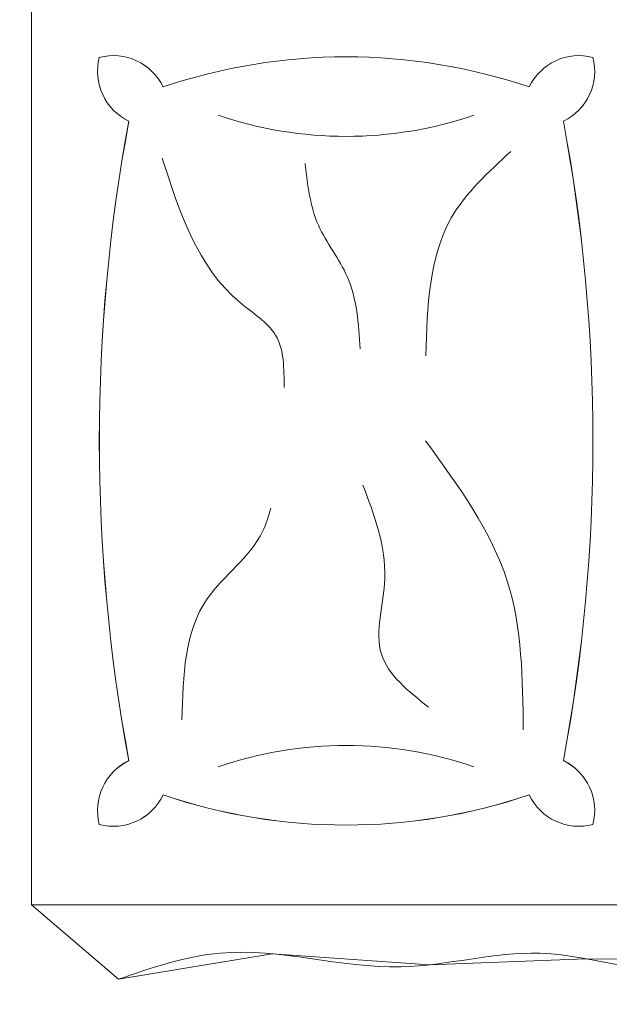
# Model space of a CAD drawing. Units: inches. Extents: x 2083 to 3317, y 1141 to 2115.
# Tile 5 of 256: x 2241 to 2260, y 1296 to 1327. Entities that reach past the tile are written whole.
import ezdxf

# ---------------------------------------------------------------- set-up
doc = ezdxf.new("R2010")
doc.units = ezdxf.units.IN
doc.layers.add('A-FURN', color=8, linetype='Continuous', lineweight=18)
doc.layers.add('www.cadblocksfree.com', color=7, linetype='Continuous', lineweight=9)
doc.layers.add('A-WALL-PATT', color=251, linetype='Continuous', lineweight=13, true_color=0x636466)

# ---------------------------------------------------------------- blocks, each defined once
blk = doc.blocks.new('bed')
at = {"layer": 'www.cadblocksfree.com', "ltscale": 0.2}
blk.add_line((3363.387, 1470.154), (3360.883, 1467.22), dxfattribs=at)
blk.add_lwpolyline([(3426.379, 1449.413), (3426.379, 1470.154), (3363.387, 1470.154), (3363.387, 1447.076)], dxfattribs=at)
for centre, radius, start, end in [((3367.903, 1467.396), 1.87, 165.5166, 244.2099), ((3366.56, 1466.054), 1.87, 25.7901, 104.4834), ((3379.014, 1409.187), 58.677, 79.42346, 100.57654), ((3391.467, 1466.054), 1.87, 75.5166, 154.2099), ((3390.125, 1467.396), 1.87, 295.7901, 14.4834), ((3385.289, 1459.547), 19.215, 161.2852, 198.7148), ((3372.739, 1459.547), 19.215, 341.2852, 18.7148), ((3355.416, 1459.547), 13.338, 341.1598, 18.8402), ((3402.612, 1459.547), 13.338, 161.1598, 198.8402), ((3367.903, 1451.698), 1.87, 115.7901, 194.4834), ((3390.125, 1451.698), 1.87, 345.5166, 64.2099), ((3366.56, 1453.041), 1.87, 255.5166, 334.2099), ((3379.014, 1509.907), 58.677, 259.42346, 280.57654), ((3391.467, 1453.041), 1.87, 205.7901, 284.4834)]:
    blk.add_arc(centre, radius, start, end, dxfattribs=at)
for points, knots in [([(3360.883, 1467.22), (3361.272, 1466.08), (3362.328, 1462.983), (3360.73, 1458.154), (3362.389, 1452.621), (3360.35, 1448.139), (3362.429, 1444.241), (3360.039, 1441.931), (3360.256, 1438.678), (3362.05, 1436.545), (3362.42, 1434.517), (3362.566, 1432.758), (3363.096, 1431.712), (3363.387, 1431.137)], [0, 0, 0, 0, 3.550403, 9.643115, 14.356056, 20.206026, 23.427697, 25.46537, 29.172767, 31.884544, 33.668442, 35.237641, 37.145618, 37.145618, 37.145618, 37.145618]), ([(3388.545, 1465.744), (3386.719, 1465.161), (3384.357, 1464.407), (3382.678, 1461.635), (3381.454, 1461.638), (3380.813, 1461.64)], [0, 0, 0, 0, 5.530688, 7.154877, 8.940839, 8.940839, 8.940839, 8.940839]), ([(3369.625, 1465.083), (3371.104, 1465.041), (3373.625, 1464.969), (3375.264, 1462.52), (3376.483, 1462.165), (3376.755, 1462.086)], [0, 0, 0, 0, 4.163459, 7.093919, 7.934624, 7.934624, 7.934624, 7.934624]), ([(3388.358, 1460.927), (3387.639, 1460.846), (3386.254, 1460.689), (3384.483, 1459.224), (3382.96, 1459.127), (3382.112, 1459.073)], [0, 0, 0, 0, 2.127543, 4.10272, 6.58647, 6.58647, 6.58647, 6.58647]), ([(3370.049, 1456.774), (3370.592, 1457.459), (3371.713, 1458.876), (3374.682, 1457.893), (3376.505, 1458.594), (3377.525, 1458.985)], [0, 0, 0, 0, 2.388143, 4.935423, 8.166198, 8.166198, 8.166198, 8.166198]), ([(3369.287, 1453.579), (3370.996, 1453.599), (3374.587, 1453.639), (3377.497, 1455.762), (3379.021, 1456.874)], [0, 0, 0, 0, 5.002087, 10.507046, 10.507046, 10.507046, 10.507046]), ([(3388.77, 1453.995), (3388.068, 1454.761), (3386.268, 1456.726), (3383.544, 1456.811), (3381.881, 1456.863)], [0, 0, 0, 0, 3.013696, 7.735839, 7.735839, 7.735839, 7.735839])]:
    blk.add_open_spline(points, degree=3, knots=knots, dxfattribs=at)

msp = doc.modelspace()

# ---------------------------------------------------------------- hatches: boundary and pattern name
at = {"layer": 'A-WALL-PATT'}
h = msp.add_hatch(color=256, dxfattribs=at)
h.dxf.hatch_style = 1
h.paths.add_polyline_path([(3126.96, 2020.761), (2748.96, 2020.761), (2604.96, 2020.761), (2226.96, 2020.761), (2226.96, 1702.761), (2466.96, 1702.761), (2466.96, 1582.761), (2418.96, 1582.761), (2418.96, 1477.761), (2226.96, 1477.761), (2226.96, 1263.261), (2544.96, 1263.261), (2544.96, 1411.761), (2604.96, 1411.761), (2685.96, 1411.761), (2685.96, 1420.761), (2604.96, 1420.761), (2604.96, 1573.761), (2604.96, 1702.761), (2604.96, 2011.761), (2748.96, 2011.761), (2748.96, 1702.761), (2862.96, 1702.761), (2862.96, 1621.761), (2871.96, 1621.761), (2871.96, 1702.761), (2883.96, 1702.761), (2883.96, 1706.939, -0.026459), (2883.96, 1711.761), (2757.96, 1711.761), (2757.96, 1807.761), (2787.96, 1807.761), (2787.96, 1812.261), (2757.96, 1812.261), (2757.96, 2011.761), (2877.96, 2011.761), (2877.96, 1812.261), (2847.96, 1812.261), (2847.96, 1807.761), (2889.836, 1807.761), (2889.836, 1812.261), (2882.46, 1812.261), (2882.46, 2011.761), (3117.96, 2011.761), (3117.96, 1812.261), (2937.836, 1812.261), (2937.836, 1807.761), (2995.71, 1807.761), (2995.71, 1796.118), (3000.21, 1796.118), (3000.21, 1807.761), (3117.96, 1807.761), (3117.96, 1711.761), (3000.21, 1711.761), (3000.21, 1760.118), (2998.573, 1760.118, -0.020711), (2995.71, 1760.118), (2995.71, 1711.761), (2931.96, 1711.761), (2931.96, 1702.761), (3126.96, 1702.761)])
h.paths.add_polyline_path([(2471.46, 2011.761), (2471.46, 1810.011), (2462.717, 1810.011), (2462.717, 1805.511), (2505.96, 1805.511), (2505.96, 1810.011), (2475.96, 1810.011), (2475.96, 2011.761), (2595.96, 2011.761), (2595.96, 1810.011), (2565.96, 1810.011), (2565.96, 1805.511), (2595.96, 1805.511), (2595.96, 1711.761), (2235.96, 1711.761), (2235.96, 1805.511), (2353.71, 1805.511), (2353.71, 1796.054), (2358.21, 1796.054), (2358.21, 1805.511), (2414.717, 1805.511), (2414.717, 1810.011), (2235.96, 1810.011), (2235.96, 2011.761)], flags=16)
h.paths.add_polyline_path([(2270.205, 1994.61), (2270.205, 1970.61), (2246.205, 1970.61), (2246.205, 1994.61)], flags=0)
edge = h.paths.add_edge_path(flags=0)
edge.add_ellipse((2332.027, 1899.798), major_axis=(-3.043, 3.043), ratio=0.168252, start_angle=-161.3322, end_angle=-156.3071, ccw=False)
edge.add_ellipse((2333.082, 1898.744), major_axis=(-1.055, 1.055), ratio=0.453532, start_angle=-123.371, end_angle=-94.1591)
edge = h.paths.add_edge_path(flags=0)
edge.add_ellipse((2332.027, 1968.876), major_axis=(3.043, 3.043), ratio=0.168252, start_angle=18.6678, end_angle=23.6929)
edge.add_spline(control_points=[(2332.926, 1970.691), (2332.227, 1970.336), (2330.894, 1969.659), (2328.413, 1970.932), (2327.204, 1967.749), (2324.71, 1969.956), (2322.533, 1967.012), (2320.013, 1971.296), (2317.68, 1968.158), (2316.041, 1967.102), (2315.427, 1966.81)], knot_values=[0, 0, 0, 0, 2.267059, 4.324559, 6.685584, 8.878641, 11.121502, 14.300359, 17.755284, 19.732645, 19.732645, 19.732645, 19.732645], degree=3, periodic=0)
edge.add_ellipse((2332.027, 1968.876), major_axis=(3.043, 3.043), ratio=0.168252, start_angle=18.6678, end_angle=23.6929, ccw=False)
edge.add_ellipse((2333.082, 1969.931), major_axis=(1.055, 1.055), ratio=0.453532, start_angle=56.629, end_angle=85.8409, ccw=False)
edge = h.paths.add_edge_path(flags=0)
edge.add_spline(control_points=[(2296.428, 1967.988), (2293.628, 1965.336), (2287.704, 1959.727), (2299.744, 1949.996), (2294.533, 1935.669), (2290.573, 1920.604), (2293.394, 1909.974), (2296.185, 1904.967)], knot_values=[0.099185, 0.099185, 0.099185, 0.099185, 0.345301, 0.619822, 0.982653, 1.386093, 1.810555, 1.810555, 1.810555, 1.810555], degree=3, periodic=0)
edge.add_spline(control_points=[(2296.185, 1904.967), (2297.384, 1902.619), (2298.001, 1901.949), (2298.553, 1901.468)], knot_values=[0.006246, 0.006246, 0.006246, 0.006246, 0.055476, 0.055476, 0.055476, 0.055476], degree=3, periodic=0)
edge.add_spline(control_points=[(2298.553, 1901.468), (2297.259, 1900.923), (2295.225, 1900.232), (2293.06, 1900.614), (2292.101, 1900.788), (2292.09, 1900.791)], knot_values=[0.312835, 0.312835, 0.312835, 0.312835, 0.40178, 0.474987, 0.475903, 0.475903, 0.475903, 0.475903], degree=3, periodic=0)
edge.add_arc((2292.794, 1904.664), 3.937, 215.4209, 259.6982, ccw=False)
edge.add_spline(control_points=[(2289.585, 1902.382), (2289.477, 1902.535), (2289.368, 1902.688), (2289.261, 1902.841)], knot_values=[0.102872, 0.102872, 0.102872, 0.102872, 0.116896, 0.116896, 0.116896, 0.116896], degree=3, periodic=0)
edge.add_spline(control_points=[(2289.261, 1902.841), (2288.687, 1902.55), (2287.64, 1902.02), (2285.881, 1901.874), (2283.853, 1901.504), (2281.72, 1899.711), (2278.467, 1899.493), (2276.157, 1901.883), (2272.259, 1899.804), (2267.778, 1901.843), (2262.244, 1900.184), (2257.415, 1901.782), (2254.318, 1900.726), (2253.178, 1900.337)], knot_values=[0, 0, 0, 0, 1.907977, 3.477176, 5.261074, 7.972851, 11.680248, 13.717921, 16.939592, 22.789562, 27.502503, 33.595215, 37.145618, 37.145618, 37.145618, 37.145618], degree=3, periodic=0)
edge.add_line((2253.178, 1900.337), (2250.244, 1902.841))
edge.add_line((2250.244, 1902.841), (2250.244, 1965.833))
edge.add_line((2250.244, 1965.833), (2253.178, 1968.337))
edge.add_spline(control_points=[(2253.178, 1968.337), (2254.318, 1967.948), (2257.415, 1966.892), (2262.244, 1968.49), (2267.778, 1966.831), (2271.527, 1968.537), (2273.876, 1967.828), (2274.207, 1967.728)], knot_values=[0, 0, 0, 0, 0.09018, 0.244935, 0.364644, 0.513233, 0.537855, 0.537855, 0.537855, 0.537855], degree=3, periodic=0)
edge.add_arc((2274.353, 1963.793), 3.937, 72.0511, 92.1279, ccw=False)
edge.add_arc((2281.297, 1985.23), 18.596, 252.0511, 288.5657)
edge.add_arc((2292.317, 1956.029), 12.646, 71.0268, 113.7782, ccw=False)
edge = h.paths.add_edge_path(flags=0)
edge.add_spline(control_points=[(2274.899, 1951.856), (2275.066, 1951.617), (2275.233, 1951.377), (2275.398, 1951.136)], knot_values=[1.409916, 1.409916, 1.409916, 1.409916, 1.43159, 1.43159, 1.43159, 1.43159], degree=3, periodic=0)
edge.add_spline(control_points=[(2275.398, 1951.136), (2275.792, 1950.562), (2276.179, 1949.984), (2276.546, 1949.397)], knot_values=[1.358238, 1.358238, 1.358238, 1.358238, 1.409916, 1.409916, 1.409916, 1.409916], degree=3, periodic=0)
edge.add_line((2276.546, 1949.397), (2277.437, 1947.862))
edge.add_spline(control_points=[(2277.437, 1947.862), (2276.304, 1945.673), (2274.64, 1942.427), (2274.632, 1938.094), (2272.799, 1930.852), (2274.356, 1943.897), (2275.948, 1947.923), (2276.546, 1949.397)], knot_values=[0.005632, 0.005632, 0.005632, 0.005632, 0.186014, 0.266002, 0.357087, 0.59639, 0.739732, 0.739732, 0.739732, 0.739732], degree=3, periodic=0)
edge.add_spline(control_points=[(2276.546, 1949.397), (2276.179, 1949.984), (2275.792, 1950.562), (2275.398, 1951.136)], knot_values=[1.358238, 1.358238, 1.358238, 1.358238, 1.409916, 1.409916, 1.409916, 1.409916], degree=3, periodic=0)
edge.add_spline(control_points=[(2275.398, 1951.136), (2274.943, 1950.08), (2274.208, 1948.025), (2273.935, 1944.851), (2272.469, 1937.627), (2273.466, 1945.696), (2274.701, 1951.059), (2274.899, 1951.856)], knot_values=[0.104364, 0.104364, 0.104364, 0.104364, 0.189636, 0.269624, 0.36071, 0.600013, 0.644622, 0.644622, 0.644622, 0.644622], degree=3, periodic=0)
h.paths.add_polyline_path([(2269.168, 1963.128, -0.357527), (2268.171, 1960.976, -0.092561), (2268.171, 1939.436, -0.357527), (2269.168, 1937.285, -0.357527), (2267.016, 1938.282, -0.164785), (2254.686, 1938.282, -0.357527), (2252.534, 1937.285, -0.357527), (2253.531, 1939.436, -0.092561), (2253.531, 1960.976, -0.357527), (2252.534, 1963.128, -0.357527), (2254.686, 1962.131, -0.164785), (2267.016, 1962.131, -0.357527)], flags=0)
h.paths.add_polyline_path([(2248.874, 1967.802), (2248.874, 1957.028), (2249.458, 1957.028), (2249.458, 1911.647), (2248.874, 1911.647), (2248.874, 1900.873), (2246.512, 1900.873, 0.197327), (2244.15, 1902.457), (2244.15, 1966.218, 0.197327), (2246.512, 1967.802)], flags=0)
h.paths.add_polyline_path([(2269.168, 1931.389, -0.357527), (2268.171, 1929.238, -0.092561), (2268.171, 1907.698, -0.357527), (2269.168, 1905.547, -0.357527), (2267.016, 1906.544, -0.164785), (2254.686, 1906.544, -0.357527), (2252.534, 1905.547, -0.357527), (2253.531, 1907.698, -0.092561), (2253.531, 1929.238, -0.357527), (2252.534, 1931.389, -0.357527), (2254.686, 1930.392, -0.164785), (2267.016, 1930.392, -0.357527)], flags=0)
edge = h.paths.add_edge_path(flags=0)
edge.add_spline(control_points=[(2276.197, 1906.724), (2276.168, 1909.029), (2276.114, 1913.372), (2270.598, 1924.925), (2273.905, 1919.013), (2275.922, 1916.262), (2275.475, 1912.402), (2277.258, 1910.381), (2276.696, 1908.225), (2276.646, 1906.813), (2276.618, 1906.008)], knot_values=[0, 0, 0, 0, 8.61026, 16.221274, 18.843057, 23.804898, 27.440828, 29.356102, 31.203478, 33.650687, 33.650687, 33.650687, 33.650687], degree=3, periodic=0)
edge.add_spline(control_points=[(2276.618, 1906.008), (2276.623, 1905.624), (2276.498, 1904.629), (2275.442, 1903.855), (2274.937, 1903.08), (2274.859, 1902.841)], knot_values=[0.156488, 0.156488, 0.156488, 0.156488, 0.184398, 0.231376, 0.250598, 0.250598, 0.250598, 0.250598], degree=3, periodic=0)
edge.add_line((2274.859, 1902.841), (2276.506, 1902.841))
edge.add_spline(control_points=[(2276.506, 1902.841), (2276.788, 1903.085), (2277.665, 1904.125), (2278.25, 1904.341), (2277.654, 1908.527), (2278.156, 1906.228), (2278.1, 1905.286), (2278.847, 1904.069), (2277.857, 1903.415), (2277.874, 1902.991), (2277.904, 1902.841)], knot_values=[0.059574, 0.059574, 0.059574, 0.059574, 0.080753, 0.103741, 0.16972, 0.176036, 0.207137, 0.240474, 0.262341, 0.27366, 0.27366, 0.27366, 0.27366], degree=3, periodic=0)
edge.add_line((2277.904, 1902.841), (2280.03, 1902.841))
edge.add_spline(control_points=[(2280.03, 1902.841), (2279.888, 1903.088), (2279.499, 1903.982), (2280.152, 1905.939), (2278.104, 1909.658), (2279.762, 1907.185), (2280.328, 1904.875), (2280.485, 1903.49), (2281.463, 1903.249), (2281.758, 1902.936), (2281.834, 1902.841)], knot_values=[0.013856, 0.013856, 0.013856, 0.013856, 0.034874, 0.088867, 0.107879, 0.126738, 0.158714, 0.193757, 0.217487, 0.226722, 0.226722, 0.226722, 0.226722], degree=3, periodic=0)
edge.add_spline(control_points=[(2281.834, 1902.841), (2281.788, 1902.827), (2281.647, 1902.783), (2281.396, 1902.859), (2281.088, 1902.985), (2280.721, 1903.061), (2280.333, 1903.026), (2280.125, 1902.899), (2280.03, 1902.841)], knot_values=[0, 0, 0, 0, 0.14413, 0.435517, 0.749276, 1.153046, 1.548371, 1.878348, 1.878348, 1.878348, 1.878348], degree=3, periodic=0)
edge.add_line((2280.03, 1902.841), (2277.904, 1902.841))
edge.add_spline(control_points=[(2277.904, 1902.841), (2277.893, 1902.796), (2277.865, 1902.68), (2277.607, 1902.687), (2277.274, 1902.801), (2276.838, 1902.62), (2276.584, 1902.789), (2276.506, 1902.841)], knot_values=[0, 0, 0, 0, 0.127189, 0.326199, 0.628009, 1.24357, 1.515331, 1.515331, 1.515331, 1.515331], degree=3, periodic=0)
edge.add_line((2276.506, 1902.841), (2274.859, 1902.841))
edge.add_spline(control_points=[(2274.859, 1902.841), (2274.814, 1902.899), (2274.725, 1903.013), (2274.493, 1903.119), (2274.244, 1902.961), (2273.937, 1903.185), (2273.614, 1902.983), (2273.408, 1902.883), (2273.322, 1902.841)], knot_values=[0, 0, 0, 0, 0.21843, 0.436957, 0.687977, 0.990379, 1.398396, 1.69185, 1.69185, 1.69185, 1.69185], degree=3, periodic=0)
edge.add_spline(control_points=[(2273.322, 1902.841), (2273.617, 1903.446), (2274.274, 1904.538), (2276.027, 1904.574), (2276.207, 1906.584), (2276.197, 1906.724)], knot_values=[0.012227, 0.012227, 0.012227, 0.012227, 0.059472, 0.106218, 0.134458, 0.134458, 0.134458, 0.134458], degree=3, periodic=0)
h.paths.add_polyline_path([(2270.776, 1897.79), (2270.776, 1873.79), (2246.776, 1873.79), (2246.776, 1897.79)], flags=0)
h.paths.add_polyline_path([(2353.71, 1760.005), (2353.71, 1760.054), (2358.21, 1760.054, -0.033729)], flags=0)
h.paths.add_polyline_path([(2321.819, 1737.529), (2341.995, 1737.529, -0.414214), (2343.203, 1736.321), (2343.203, 1721.021, -0.414214), (2341.995, 1719.813), (2321.819, 1719.813, -0.414214), (2320.611, 1721.021), (2320.611, 1736.321, -0.414214)], flags=0)
h.paths.add_polyline_path([(2324.235, 1736.321), (2339.579, 1736.321, -0.414214), (2341.995, 1733.905), (2341.995, 1725.45, -0.414214), (2339.579, 1723.034), (2333.681, 1723.034), (2333.845, 1722.045, -0.870646), (2335.425, 1721.826, -0.767327), (2333.923, 1721.423), (2331.291, 1721.423, -0.767327), (2329.788, 1721.826, -0.870646), (2331.368, 1722.045), (2331.533, 1723.034), (2324.235, 1723.034, -0.414214), (2321.819, 1725.45), (2321.819, 1733.905, -0.414214)], flags=0)
h.paths.add_polyline_path([(2570.484, 1928.615), (2589.684, 1928.615), (2590.169, 1928.615), (2590.169, 1904.993), (2570.484, 1904.993)], flags=0)
h.paths.add_polyline_path([(2574.447, 1927.264, -1), (2572.829, 1927.264, -1)], flags=0)
h.paths.add_polyline_path([(2573.09, 1926.941), (2573.925, 1927.776), (2574.148, 1927.553), (2573.313, 1926.718)], flags=0)
h.paths.add_polyline_path([(2578.779, 1919.73, -1), (2571.592, 1919.73, -1)], flags=0)
h.paths.add_polyline_path([(2578.385, 1919.73, -1), (2571.985, 1919.73, -1)], flags=0)
h.paths.add_polyline_path([(2331.596, 1729.476, -1), (2333.618, 1729.476, -1)], flags=0)
h.paths.add_polyline_path([(2578.034, 1927.264, -1), (2576.416, 1927.264, -1)], flags=0)
h.paths.add_polyline_path([(2576.689, 1927.531), (2576.912, 1927.754), (2577.747, 1926.919), (2577.524, 1926.696)], flags=0)
h.paths.add_polyline_path([(2578.139, 1909.86, -1), (2572.232, 1909.86, -1)], flags=0)
h.paths.add_polyline_path([(2577.745, 1909.86, -1), (2572.625, 1909.86, -1)], flags=0)
h.paths.add_polyline_path([(2583.798, 1927.264, -1), (2582.179, 1927.264, -1)], flags=0)
h.paths.add_polyline_path([(2582.719, 1927.754), (2583.554, 1926.919), (2583.331, 1926.696), (2582.496, 1927.531)], flags=0)
h.paths.add_polyline_path([(2582.496, 1927.531), (2582.719, 1927.754), (2583.554, 1926.919), (2583.331, 1926.696)], flags=0)
h.paths.add_polyline_path([(2587.739, 1920.53, -1), (2581.832, 1920.53, -1)], flags=0)
h.paths.add_polyline_path([(2587.345, 1920.53, -1), (2582.225, 1920.53, -1)], flags=0)
h.paths.add_polyline_path([(2587.385, 1927.264, -1), (2585.766, 1927.264, -1)], flags=0)
h.paths.add_polyline_path([(2586.082, 1926.98), (2586.917, 1927.815), (2587.14, 1927.593), (2586.305, 1926.758)], flags=0)
h.paths.add_polyline_path([(2588.379, 1910.66, -1), (2581.192, 1910.66, -1)], flags=0)
h.paths.add_polyline_path([(2587.985, 1910.66, -1), (2581.585, 1910.66, -1)], flags=0)
h.paths.add_polyline_path([(2417.168, 1729.478), (2437.344, 1729.478, -0.414214), (2438.552, 1728.27), (2438.552, 1712.969, -0.414214), (2437.344, 1711.761), (2417.168, 1711.761, -0.414214), (2415.96, 1712.969), (2415.96, 1728.27, -0.414214)], flags=0)
h.paths.add_polyline_path([(2419.584, 1728.27), (2434.928, 1728.27, -0.414214), (2437.344, 1725.854), (2437.344, 1717.398, -0.414214), (2434.928, 1714.983), (2429.029, 1714.983), (2429.194, 1713.994, -0.870646), (2430.774, 1713.775, -0.767327), (2429.271, 1713.372), (2426.64, 1713.372, -0.767327), (2425.137, 1713.775, -0.870646), (2426.717, 1713.994), (2426.882, 1714.983), (2419.584, 1714.983, -0.414214), (2417.168, 1717.398), (2417.168, 1725.854, -0.414214)], flags=0)
h.paths.add_polyline_path([(2419.584, 1728.27), (2434.928, 1728.27, -0.414214), (2437.344, 1725.854), (2437.344, 1717.398, -0.414214), (2434.928, 1714.983), (2429.029, 1714.983), (2428.358, 1719.009), (2427.553, 1719.009), (2426.882, 1714.983), (2419.584, 1714.983, -0.414214), (2417.168, 1717.398), (2417.168, 1725.854, -0.414214)], flags=0)
h.paths.add_polyline_path([(2426.944, 1721.425, -1), (2428.967, 1721.425, -1)], flags=0)
h.paths.add_polyline_path([(2475.96, 1702.761), (2595.96, 1702.761), (2595.96, 1582.761), (2475.96, 1582.761)], flags=16)
h.paths.add_polyline_path([(2427.96, 1573.761), (2595.96, 1573.761), (2595.96, 1468.761), (2595.96, 1420.761), (2384.46, 1420.761), (2384.46, 1468.761), (2427.96, 1468.761)], flags=16)
h.paths.add_polyline_path([(2379.96, 1468.761), (2379.96, 1420.761), (2235.96, 1420.761), (2235.96, 1468.761)], flags=16)
h.paths.add_polyline_path([(2317.816, 1466.696), (2337.992, 1466.696, -0.414214), (2339.2, 1465.488), (2339.2, 1450.187, -0.414214), (2337.992, 1448.979), (2317.816, 1448.979, -0.414214), (2316.608, 1450.187), (2316.608, 1465.488, -0.414214)], flags=0)
h.paths.add_polyline_path([(2320.232, 1465.488), (2335.576, 1465.488, -0.414214), (2337.992, 1463.072), (2337.992, 1454.616, -0.414214), (2335.576, 1452.2), (2329.677, 1452.2), (2329.842, 1451.212, -0.870646), (2331.422, 1450.992, -0.767327), (2329.92, 1450.59), (2327.288, 1450.59, -0.767327), (2325.785, 1450.992, -0.870646), (2327.365, 1451.212), (2327.53, 1452.2), (2320.232, 1452.2, -0.414214), (2317.816, 1454.616), (2317.816, 1463.072, -0.414214)], flags=0)
h.paths.add_polyline_path([(2320.232, 1465.488), (2335.576, 1465.488, -0.414214), (2337.992, 1463.072), (2337.992, 1454.616, -0.414214), (2335.576, 1452.2), (2329.677, 1452.2), (2329.006, 1456.227), (2328.201, 1456.227), (2327.53, 1452.2), (2320.232, 1452.2, -0.414214), (2317.816, 1454.616), (2317.816, 1463.072, -0.414214)], flags=0)
h.paths.add_polyline_path([(2327.593, 1458.643, -1), (2329.615, 1458.643, -1)], flags=0)
h.paths.add_polyline_path([(2244.412, 1433.34), (2241.921, 1433.34, -0.414214), (2240.018, 1435.244), (2240.018, 1440.953, -0.414211), (2241.921, 1442.856), (2244.412, 1442.856, -1.976472)], flags=0)
h.paths.add_polyline_path([(2245.357, 1434.398, -0.414214), (2245.357, 1441.799, -2.144098)], flags=0)
h.paths.add_polyline_path([(2535.96, 1416.261), (2535.96, 1272.261), (2235.96, 1272.261), (2235.96, 1416.261)], flags=16)
h.paths.add_polyline_path([(2260.12, 1384.293), (2260.12, 1362.039), (2237.865, 1362.039), (2237.865, 1384.293)], flags=0)
edge = h.paths.add_edge_path(flags=0)
edge.add_line((2318.252, 1362.093), (2318.146, 1362.001))
edge.add_ellipse((2317.445, 1360.431), major_axis=(2.822, 2.822), ratio=0.168252, start_angle=18.6678, end_angle=20.9481, ccw=False)
edge.add_ellipse((2318.423, 1361.409), major_axis=(0.978, 0.978), ratio=0.453532, start_angle=56.629, end_angle=70.2262, ccw=False)
edge = h.paths.add_edge_path(flags=0)
edge.add_line((2319.107, 1295.571), (2319.015, 1295.677))
edge.add_ellipse((2317.445, 1296.378), major_axis=(-2.822, 2.822), ratio=0.168252, start_angle=-161.3322, end_angle=-159.0519, ccw=False)
edge.add_ellipse((2318.423, 1295.4), major_axis=(-0.978, 0.978), ratio=0.453532, start_angle=-123.371, end_angle=-109.7738)
edge = h.paths.add_edge_path(flags=0)
edge.add_spline(control_points=[(2284.21, 1301.17), (2284.581, 1300.445), (2284.891, 1299.892), (2285.16, 1299.461)], knot_values=[0.039066, 0.039066, 0.039066, 0.039066, 0.055476, 0.055476, 0.055476, 0.055476], degree=3, periodic=0)
edge.add_line((2285.16, 1299.461), (2284.21, 1301.17))
edge = h.paths.add_edge_path(flags=0)
edge.add_line((2280.412, 1297.298), (2283.37, 1297.036))
edge.add_line((2283.37, 1297.036), (2286.406, 1297.926))
edge.add_spline(control_points=[(2286.406, 1297.926), (2285.305, 1297.463), (2284.345, 1297.129), (2283.37, 1297.036)], knot_values=[0.394369, 0.394369, 0.394369, 0.394369, 0.475903, 0.475903, 0.475903, 0.475903], degree=3, periodic=0)
edge.add_spline(control_points=[(2283.37, 1297.036), (2283.281, 1297.028), (2282.316, 1296.957), (2281.313, 1297.134), (2280.423, 1297.296), (2280.412, 1297.298)], knot_values=[0.312835, 0.312835, 0.312835, 0.312835, 0.320246, 0.393453, 0.394369, 0.394369, 0.394369, 0.394369], degree=3, periodic=0)
edge = h.paths.add_edge_path(flags=0)
edge.add_line((2284.436, 1359.607), (2280.446, 1355.328))
edge.add_line((2280.446, 1355.328), (2279.58, 1351.018))
edge.add_line((2279.58, 1351.018), (2282.413, 1346.58))
edge.add_spline(control_points=[(2282.413, 1346.58), (2283.153, 1345.589), (2284.253, 1344.029), (2284.801, 1342.387), (2284.935, 1341.806)], knot_values=[1.240098, 1.240098, 1.240098, 1.240098, 1.332892, 1.382712, 1.382712, 1.382712, 1.382712], degree=3, periodic=0)
edge.add_spline(control_points=[(2284.935, 1341.806), (2285.319, 1340.141), (2285.233, 1338.409), (2284.91, 1336.654)], knot_values=[1.097484, 1.097484, 1.097484, 1.097484, 1.240098, 1.240098, 1.240098, 1.240098], degree=3, periodic=0)
edge.add_spline(control_points=[(2284.91, 1336.654), (2284.587, 1334.899), (2284.027, 1333.12), (2283.463, 1331.361)], knot_values=[0.95487, 0.95487, 0.95487, 0.95487, 1.097484, 1.097484, 1.097484, 1.097484], degree=3, periodic=0)
edge.add_line((2283.463, 1331.361), (2281.89, 1326.153))
edge.add_line((2281.89, 1326.153), (2280.756, 1321.056))
edge.add_line((2280.756, 1321.056), (2280.299, 1316.002))
edge.add_line((2280.299, 1316.002), (2280.716, 1310.95))
edge.add_line((2280.716, 1310.95), (2282.028, 1305.972))
edge.add_line((2282.028, 1305.972), (2284.21, 1301.17))
edge.add_spline(control_points=[(2284.21, 1301.17), (2283.341, 1302.73), (2282.612, 1304.336), (2282.028, 1305.972)], knot_values=[0.099185, 0.099185, 0.099185, 0.099185, 0.241799, 0.241799, 0.241799, 0.241799], degree=3, periodic=0)
edge.add_spline(control_points=[(2282.028, 1305.972), (2281.444, 1307.608), (2281.005, 1309.273), (2280.716, 1310.95)], knot_values=[0.241799, 0.241799, 0.241799, 0.241799, 0.384413, 0.384413, 0.384413, 0.384413], degree=3, periodic=0)
edge.add_spline(control_points=[(2280.716, 1310.95), (2280.433, 1312.588), (2280.289, 1314.277), (2280.299, 1315.962), (2280.299, 1316.002)], knot_values=[0.384413, 0.384413, 0.384413, 0.384413, 0.523647, 0.527028, 0.527028, 0.527028, 0.527028], degree=3, periodic=0)
edge.add_spline(control_points=[(2280.299, 1316.002), (2280.312, 1317.687), (2280.478, 1319.368), (2280.756, 1321.056)], knot_values=[0.527028, 0.527028, 0.527028, 0.527028, 0.669642, 0.669642, 0.669642, 0.669642], degree=3, periodic=0)
edge.add_spline(control_points=[(2280.756, 1321.056), (2281.035, 1322.744), (2281.426, 1324.44), (2281.89, 1326.153)], knot_values=[0.669642, 0.669642, 0.669642, 0.669642, 0.812256, 0.812256, 0.812256, 0.812256], degree=3, periodic=0)
edge.add_spline(control_points=[(2281.89, 1326.153), (2282.264, 1327.533), (2282.788, 1329.262), (2283.353, 1331.018), (2283.463, 1331.361)], knot_values=[0.812256, 0.812256, 0.812256, 0.812256, 0.927087, 0.95487, 0.95487, 0.95487, 0.95487], degree=3, periodic=0)
edge.add_line((2283.463, 1331.361), (2284.91, 1336.654))
edge.add_line((2284.91, 1336.654), (2284.935, 1341.806))
edge.add_line((2284.935, 1341.806), (2282.413, 1346.58))
edge.add_spline(control_points=[(2282.413, 1346.58), (2281.275, 1348.104), (2280.078, 1349.57), (2279.58, 1351.018)], knot_values=[1.382712, 1.382712, 1.382712, 1.382712, 1.525326, 1.525326, 1.525326, 1.525326], degree=3, periodic=0)
edge.add_spline(control_points=[(2279.58, 1351.018), (2279.443, 1351.415), (2279.136, 1352.857), (2279.735, 1354.29), (2280.446, 1355.328)], knot_values=[1.525326, 1.525326, 1.525326, 1.525326, 1.564439, 1.667941, 1.667941, 1.667941, 1.667941], degree=3, periodic=0)
edge.add_spline(control_points=[(2280.446, 1355.328), (2281.426, 1356.758), (2282.931, 1358.183), (2284.436, 1359.607)], knot_values=[1.667941, 1.667941, 1.667941, 1.667941, 1.810555, 1.810555, 1.810555, 1.810555], degree=3, periodic=0)
edge.add_arc((2280.623, 1348.518), 11.726, 71.0268, 113.7782)
edge.add_arc((2270.405, 1375.595), 17.244, 252.0511, 288.5657, ccw=False)
edge.add_arc((2263.966, 1355.718), 3.651, 72.0511, 92.1279)
edge.add_arc((2263.966, 1355.718), 3.651, 92.1279, 177.9851)
edge.add_spline(control_points=[(2260.318, 1355.846), (2260.26, 1354.221), (2260.551, 1350.187), (2262.999, 1346.766), (2264.473, 1344.649)], knot_values=[1.43159, 1.43159, 1.43159, 1.43159, 1.564144, 1.770695, 1.770695, 1.770695, 1.770695], degree=3, periodic=0)
edge.add_line((2264.473, 1344.649), (2264.936, 1343.983))
edge.add_spline(control_points=[(2263.801, 1340.248), (2263.843, 1340.514), (2264.067, 1341.756), (2264.513, 1343.002), (2264.935, 1343.981)], knot_values=[0.53657, 0.53657, 0.53657, 0.53657, 0.559349, 0.644622, 0.644622, 0.644622, 0.644622], degree=3, periodic=0)
edge.add_spline(control_points=[(2264.935, 1343.981), (2265.118, 1343.715), (2265.299, 1343.448), (2265.477, 1343.179)], knot_values=[1.384077, 1.384077, 1.384077, 1.384077, 1.409916, 1.409916, 1.409916, 1.409916], degree=3, periodic=0)
edge.add_spline(control_points=[(2265.477, 1343.179), (2265.655, 1342.911), (2265.829, 1342.641), (2265.999, 1342.369)], knot_values=[1.358238, 1.358238, 1.358238, 1.358238, 1.384077, 1.384077, 1.384077, 1.384077], degree=3, periodic=0)
edge.add_line((2265.999, 1342.369), (2266.826, 1340.946))
edge.add_spline(control_points=[(2266.826, 1340.946), (2268.894, 1337.09), (2271.398, 1325.843), (2270.516, 1310.569), (2275.919, 1301.861), (2277.79, 1299.199)], knot_values=[0.116896, 0.116896, 0.116896, 0.116896, 0.472987, 1.050969, 1.313793, 1.313793, 1.313793, 1.313793], degree=3, periodic=0)
edge.add_spline(control_points=[(2277.79, 1299.199), (2277.839, 1299.128), (2277.889, 1299.057), (2277.94, 1298.987)], knot_values=[0.109884, 0.109884, 0.109884, 0.109884, 0.116896, 0.116896, 0.116896, 0.116896], degree=3, periodic=0)
edge.add_line((2277.94, 1298.987), (2277.789, 1299.199))
edge.add_spline(control_points=[(2277.789, 1299.199), (2277.257, 1298.929), (2276.286, 1298.438), (2275.039, 1298.334), (2274.383, 1298.239), (2274.215, 1298.209)], knot_values=[33.12187, 33.12187, 33.12187, 33.12187, 35.029056, 36.598255, 37.144827, 37.144827, 37.144827, 37.144827], degree=3, periodic=0)
edge.add_line((2274.215, 1298.209), (2273.073, 1297.893))
edge.add_spline(control_points=[(2273.073, 1297.893), (2272.323, 1297.58), (2271.039, 1296.511), (2269.248, 1296.226), (2268.423, 1296.375)], knot_values=[26.532584, 26.532584, 26.532584, 26.532584, 29.198919, 31.839101, 31.839101, 31.839101, 31.839101], degree=3, periodic=0)
edge.add_line((2268.423, 1296.375), (2263.879, 1297.458))
edge.add_spline(control_points=[(2263.879, 1297.458), (2263.556, 1297.359), (2261.86, 1296.839), (2260.239, 1297.282), (2258.933, 1297.516)], knot_values=[15.919551, 15.919551, 15.919551, 15.919551, 16.939592, 21.226067, 21.226067, 21.226067, 21.226067], degree=3, periodic=0)
edge.add_line((2258.933, 1297.516), (2254.055, 1297.329))
edge.add_spline(control_points=[(2254.055, 1297.329), (2253.756, 1297.296), (2252.114, 1297.165), (2250.462, 1297.544), (2249.13, 1297.668)], knot_values=[5.306517, 5.306517, 5.306517, 5.306517, 6.276435, 10.613034, 10.613034, 10.613034, 10.613034], degree=3, periodic=0)
edge.add_line((2249.13, 1297.668), (2244.332, 1296.878))
edge.add_line((2244.332, 1296.878), (2241.611, 1299.199))
edge.add_line((2241.611, 1299.199), (2241.611, 1357.609))
edge.add_line((2241.611, 1357.609), (2244.332, 1359.931))
edge.add_line((2244.332, 1359.931), (2252.729, 1359.543))
edge.add_spline(control_points=[(2252.729, 1359.543), (2252.871, 1359.546), (2253.306, 1359.548), (2253.74, 1359.514), (2254.032, 1359.482)], knot_values=[0.233291, 0.233291, 0.233291, 0.233291, 0.244935, 0.268927, 0.268927, 0.268927, 0.268927], degree=3, periodic=0)
edge.add_line((2254.032, 1359.482), (2259.587, 1359.416))
edge.add_spline(control_points=[(2259.587, 1359.416), (2260.677, 1359.629), (2262.073, 1359.897), (2263.524, 1359.459), (2263.83, 1359.366)], knot_values=[0.422516, 0.422516, 0.422516, 0.422516, 0.513233, 0.537855, 0.537855, 0.537855, 0.537855], degree=3, periodic=0)
edge.add_arc((2263.966, 1355.718), 3.651, 72.0511, 92.1279, ccw=False)
edge.add_arc((2270.405, 1375.595), 17.244, 252.0511, 288.5657)
edge.add_arc((2280.623, 1348.518), 11.726, 71.0268, 113.7782, ccw=False)
h.paths.add_polyline_path([(2240.341, 1359.435), (2240.341, 1349.444), (2240.882, 1349.444), (2240.882, 1307.365), (2240.341, 1307.365), (2240.341, 1297.374), (2238.15, 1297.374, 0.197327), (2235.96, 1298.843), (2235.96, 1357.966, 0.197327), (2238.15, 1359.435)], flags=0)
h.paths.add_polyline_path([(2259.158, 1355.101, -0.357527), (2258.233, 1353.106, -0.092561), (2258.233, 1333.133, -0.357527), (2259.158, 1331.138, -0.357527), (2257.163, 1332.062, -0.164785), (2245.729, 1332.062, -0.357527), (2243.735, 1331.138, -0.357527), (2244.659, 1333.133, -0.092561), (2244.659, 1353.106, -0.357527), (2243.735, 1355.101, -0.357527), (2245.729, 1354.176, -0.164785), (2257.163, 1354.176, -0.357527)], flags=0)
edge = h.paths.add_edge_path(flags=0)
edge.add_line((2265.999, 1342.369), (2266.826, 1340.946))
edge.add_line((2266.826, 1340.946), (2265.308, 1337.814))
edge.add_line((2265.308, 1337.814), (2264.358, 1334.653))
edge.add_line((2264.358, 1334.653), (2264.262, 1333.8))
edge.add_spline(control_points=[(2264.262, 1333.8), (2264.208, 1333.187), (2264.162, 1332.366), (2264.007, 1331.414), (2263.969, 1331.202)], knot_values=[0.464444, 0.464444, 0.464444, 0.464444, 0.516691, 0.531608, 0.531608, 0.531608, 0.531608], degree=3, periodic=0)
edge.add_spline(control_points=[(2263.969, 1331.202), (2263.775, 1330.119), (2263.424, 1328.791), (2263.257, 1328.531), (2263.234, 1328.515)], knot_values=[0.372682, 0.372682, 0.372682, 0.372682, 0.44885, 0.464444, 0.464444, 0.464444, 0.464444], degree=3, periodic=0)
edge.add_spline(control_points=[(2263.234, 1328.515), (2263.096, 1328.42), (2263.131, 1329.301), (2263.275, 1330.616)], knot_values=[0.280919, 0.280919, 0.280919, 0.280919, 0.372682, 0.372682, 0.372682, 0.372682], degree=3, periodic=0)
edge.add_spline(control_points=[(2263.275, 1330.616), (2263.419, 1331.93), (2263.672, 1333.677), (2263.97, 1335.315)], knot_values=[0.189157, 0.189157, 0.189157, 0.189157, 0.280919, 0.280919, 0.280919, 0.280919], degree=3, periodic=0)
edge.add_spline(control_points=[(2263.97, 1335.315), (2264.1, 1336.032), (2264.419, 1337.622), (2264.755, 1338.864), (2264.947, 1339.491)], knot_values=[0.097394, 0.097394, 0.097394, 0.097394, 0.137578, 0.189157, 0.189157, 0.189157, 0.189157], degree=3, periodic=0)
edge.add_spline(control_points=[(2264.947, 1339.491), (2265.29, 1340.606), (2265.644, 1341.494), (2265.999, 1342.369)], knot_values=[0.005632, 0.005632, 0.005632, 0.005632, 0.097394, 0.097394, 0.097394, 0.097394], degree=3, periodic=0)
h.paths.add_polyline_path([(2259.158, 1325.671, -0.357527), (2258.233, 1323.676, -0.092561), (2258.233, 1303.703, -0.357527), (2259.158, 1301.708, -0.357527), (2257.163, 1302.633, -0.164785), (2245.729, 1302.633, -0.357527), (2243.735, 1301.708, -0.357527), (2244.659, 1303.703, -0.092561), (2244.659, 1323.676, -0.357527), (2243.735, 1325.671, -0.357527), (2245.729, 1324.747, -0.164785), (2257.163, 1324.747, -0.357527)], flags=0)
edge = h.paths.add_edge_path(flags=0)
edge.add_spline(control_points=[(2261.709, 1317.311), (2261.679, 1317.418), (2261.762, 1317.389), (2262.491, 1316.09), (2262.962, 1315.301)], knot_values=[14.955861, 14.955861, 14.955861, 14.955861, 16.221274, 18.694826, 18.694826, 18.694826, 18.694826], degree=3, periodic=0)
edge.add_spline(control_points=[(2262.962, 1315.301), (2262.99, 1315.254), (2263.702, 1314.067), (2264.349, 1313.127), (2264.73, 1312.164)], knot_values=[18.694826, 18.694826, 18.694826, 18.694826, 18.843057, 22.433791, 22.433791, 22.433791, 22.433791], degree=3, periodic=0)
edge.add_spline(control_points=[(2264.73, 1312.164), (2264.876, 1311.796), (2265.177, 1310.77), (2265.143, 1309.559), (2265.248, 1308.824)], knot_values=[22.433791, 22.433791, 22.433791, 22.433791, 23.804898, 26.172756, 26.172756, 26.172756, 26.172756], degree=3, periodic=0)
edge.add_line((2265.248, 1308.824), (2265.851, 1307.172))
edge.add_spline(control_points=[(2265.851, 1307.172), (2266.065, 1306.822), (2266.384, 1306.332), (2266.424, 1305.781), (2266.42, 1305.611)], knot_values=[28.062562, 28.062562, 28.062562, 28.062562, 29.356102, 29.911721, 29.911721, 29.911721, 29.911721], degree=3, periodic=0)
edge.add_spline(control_points=[(2266.42, 1305.611), (2266.416, 1305.433), (2266.394, 1305.25), (2266.365, 1305.066)], knot_values=[29.911721, 29.911721, 29.911721, 29.911721, 30.497837, 30.497837, 30.497837, 30.497837], degree=3, periodic=0)
edge.add_line((2266.365, 1305.066), (2266.066, 1302.136))
edge.add_spline(control_points=[(2266.066, 1302.136), (2266.071, 1301.78), (2265.998, 1301.2), (2265.663, 1300.759), (2265.509, 1300.586)], knot_values=[0.156488, 0.156488, 0.156488, 0.156488, 0.184398, 0.203543, 0.203543, 0.203543, 0.203543], degree=3, periodic=0)
edge.add_line((2265.509, 1300.586), (2264.435, 1299.199))
edge.add_line((2264.435, 1299.199), (2265.962, 1299.199))
edge.add_line((2265.962, 1299.199), (2267.336, 1301.175))
edge.add_line((2267.336, 1301.175), (2267.312, 1301.986))
edge.add_spline(control_points=[(2267.312, 1301.986), (2267.261, 1302.862), (2267.16, 1303.737), (2267.271, 1303.326)], knot_values=[0.126229, 0.126229, 0.126229, 0.126229, 0.166617, 0.166617, 0.166617, 0.166617], degree=3, periodic=0)
edge.add_spline(control_points=[(2267.271, 1303.326), (2267.28, 1303.294), (2267.31, 1303.175), (2267.373, 1302.884), (2267.406, 1302.683), (2267.418, 1302.601)], knot_values=[0.166617, 0.166617, 0.166617, 0.166617, 0.16972, 0.176036, 0.180765, 0.180765, 0.180765, 0.180765], degree=3, periodic=0)
edge.add_spline(control_points=[(2267.744, 1300.988), (2267.688, 1301.151), (2267.481, 1301.657), (2267.484, 1302.145), (2267.418, 1302.601)], knot_values=[0.180765, 0.180765, 0.180765, 0.180765, 0.193767, 0.220139, 0.220139, 0.220139, 0.220139], degree=3, periodic=0)
edge.add_line((2267.418, 1302.601), (2267.744, 1300.988))
edge.add_spline(control_points=[(2267.744, 1300.988), (2267.832, 1300.732), (2267.932, 1300.31), (2267.555, 1299.975), (2267.429, 1299.829)], knot_values=[0.220139, 0.220139, 0.220139, 0.220139, 0.240474, 0.25489, 0.25489, 0.25489, 0.25489], degree=3, periodic=0)
edge.add_line((2267.429, 1299.829), (2267.258, 1299.199))
edge.add_line((2267.258, 1299.199), (2269.23, 1299.199))
edge.add_spline(control_points=[(2269.23, 1299.199), (2269.099, 1299.429), (2268.843, 1300.016), (2269.012, 1300.916), (2268.947, 1301.661)], knot_values=[0.013856, 0.013856, 0.013856, 0.013856, 0.034874, 0.067073, 0.067073, 0.067073, 0.067073], degree=3, periodic=0)
edge.add_line((2268.947, 1301.661), (2268.432, 1303.603))
edge.add_spline(control_points=[(2268.432, 1303.603), (2268.176, 1304.192), (2267.596, 1305.251), (2268.041, 1304.623), (2268.251, 1304.282)], knot_values=[0.090155, 0.090155, 0.090155, 0.090155, 0.107879, 0.120289, 0.120289, 0.120289, 0.120289], degree=3, periodic=0)
edge.add_spline(control_points=[(2268.251, 1304.282), (2268.361, 1304.105), (2269.058, 1302.918), (2269.383, 1301.59), (2269.521, 1300.776), (2269.575, 1300.556)], knot_values=[0.120289, 0.120289, 0.120289, 0.120289, 0.126738, 0.158714, 0.173506, 0.173506, 0.173506, 0.173506], degree=3, periodic=0)
edge.add_line((2269.575, 1300.556), (2270.686, 1299.421))
edge.add_spline(control_points=[(2270.686, 1299.421), (2270.767, 1299.357), (2270.838, 1299.281), (2270.903, 1299.199)], knot_values=[0.21816, 0.21816, 0.21816, 0.21816, 0.226722, 0.226722, 0.226722, 0.226722], degree=3, periodic=0)
edge.add_line((2270.937, 1299.193), (2270.903, 1299.199))
edge.add_spline(control_points=[(2270.903, 1299.199), (2270.86, 1299.186), (2270.73, 1299.146), (2270.496, 1299.216), (2270.272, 1299.308), (2270.121, 1299.348), (2270.063, 1299.36)], knot_values=[0.939174, 0.939174, 0.939174, 0.939174, 1.083304, 1.374691, 1.68845, 1.878348, 1.878348, 1.878348, 1.878348], degree=3, periodic=0)
edge.add_line((2270.063, 1299.36), (2269.23, 1299.199))
edge.add_line((2269.23, 1299.199), (2267.258, 1299.199))
edge.add_spline(control_points=[(2267.258, 1299.199), (2267.248, 1299.157), (2267.223, 1299.05), (2266.984, 1299.057), (2266.809, 1299.116), (2266.677, 1299.109), (2266.637, 1299.105)], knot_values=[0.757665, 0.757665, 0.757665, 0.757665, 0.884854, 1.083864, 1.385675, 1.515331, 1.515331, 1.515331, 1.515331], degree=3, periodic=0)
edge.add_spline(control_points=[(2266.637, 1299.105), (2266.485, 1299.089), (2266.236, 1299.017), (2266.035, 1299.151), (2265.962, 1299.199)], knot_values=[0, 0, 0, 0, 0.485905, 0.757665, 0.757665, 0.757665, 0.757665], degree=3, periodic=0)
edge.add_line((2265.962, 1299.199), (2264.435, 1299.199))
edge.add_line((2264.435, 1299.199), (2263.858, 1299.367))
edge.add_spline(control_points=[(2263.858, 1299.367), (2263.819, 1299.371), (2263.78, 1299.386), (2263.74, 1299.402)], knot_values=[0.845925, 0.845925, 0.845925, 0.845925, 0.978627, 0.978627, 0.978627, 0.978627], degree=3, periodic=0)
edge.add_line((2263.722, 1299.396), (2263.01, 1299.199))
edge.add_spline(control_points=[(2263.01, 1299.199), (2263.246, 1299.683), (2263.506, 1300.128), (2263.873, 1300.408)], knot_values=[0.012227, 0.012227, 0.012227, 0.012227, 0.052971, 0.052971, 0.052971, 0.052971], degree=3, periodic=0)
edge.add_spline(control_points=[(2263.873, 1300.408), (2263.932, 1300.453), (2264.084, 1300.553), (2264.255, 1300.624), (2264.36, 1300.665)], knot_values=[0.052971, 0.052971, 0.052971, 0.052971, 0.059472, 0.069086, 0.069086, 0.069086, 0.069086], degree=3, periodic=0)
edge.add_line((2264.36, 1300.665), (2265.142, 1301.078))
edge.add_line((2265.142, 1301.078), (2265.676, 1302.8))
edge.add_line((2265.676, 1302.8), (2265.541, 1305.704))
edge.add_line((2265.541, 1305.704), (2264.803, 1309.328))
edge.add_line((2264.803, 1309.328), (2263.041, 1314.092))
edge.add_spline(control_points=[(2263.041, 1314.092), (2262.384, 1315.671), (2261.796, 1316.998), (2261.709, 1317.311)], knot_values=[11.216896, 11.216896, 11.216896, 11.216896, 14.955861, 14.955861, 14.955861, 14.955861], degree=3, periodic=0)
h.paths.add_polyline_path([(2871.96, 1416.261), (2895.91, 1416.261), (2895.91, 1420.761), (2871.96, 1420.761), (2871.96, 1501.761), (2862.96, 1501.761), (2862.96, 1420.761), (2805.96, 1420.761), (2805.96, 1411.761), (2862.96, 1411.761), (2862.96, 1263.261), (3126.96, 1263.261), (3126.96, 1411.761), (3126.96, 1486.761), (2943.96, 1486.761), (2943.96, 1477.761), (2967.86, 1477.761), (2967.86, 1420.761), (2943.91, 1420.761), (2943.91, 1416.261), (3117.96, 1416.261), (3117.96, 1420.761), (2972.36, 1420.761), (2972.36, 1477.761), (3117.96, 1477.761), (3117.96, 1420.761), (3117.96, 1272.261), (2871.96, 1272.261)], flags=0)
h.paths.add_polyline_path([(2457.126, 1485.943), (2527.603, 1485.943), (2527.603, 1537.636), (2457.126, 1537.636)], flags=8)
h.paths.add_polyline_path([(2481.005, 1609.982), (2590.766, 1609.982), (2590.766, 1682.003), (2481.005, 1682.003)], flags=8)
h.paths.add_polyline_path([(2483.085, 1729.127), (2553.562, 1729.127), (2553.562, 1780.82), (2483.085, 1780.82)], flags=8)

# ---------------------------------------------------------------- linework, layer by layer
at = {"layer": 'A-FURN'}
for p, q in [((2241.611, 1299.199), (2241.611, 1357.609)), ((2244.332, 1296.878), (2241.611, 1299.199)), ((2249.13, 1297.668), (2244.332, 1296.878)), ((2254.055, 1297.329), (2249.13, 1297.668)), ((2258.933, 1297.516), (2254.055, 1297.329)), ((2263.879, 1297.458), (2258.933, 1297.516))]:
    msp.add_line(p, q, dxfattribs=at)
for centre, radius, start, end in [((2245.413, 1325.237), 1.734, 165.5166, 244.2099), ((2244.168, 1323.992), 1.734, 25.7901, 104.4834), ((2251.446, 1307.871), 17.818, 71.2852, 108.7148), ((2258.724, 1323.992), 1.734, 75.5166, 154.2099), ((2257.479, 1325.237), 1.734, 295.7901, 14.4834), ((2298.143, 1313.69), 54.408, 169.4235, 190.5765), ((2204.749, 1313.69), 54.408, 349.4235, 10.5765), ((2245.413, 1302.142), 1.734, 115.7901, 194.4834), ((2257.479, 1302.142), 1.734, 345.5166, 64.2099), ((2244.168, 1303.387), 1.734, 255.5166, 334.2099), ((2251.446, 1319.508), 17.818, 251.2852, 288.7148), ((2258.724, 1303.387), 1.734, 205.7901, 284.4834)]:
    msp.add_arc(centre, radius, start, end, dxfattribs=at)

# ---------------------------------------------------------------- block references
at = {"layer": 'A-FURN', "xscale": 0.9272580240292334, "yscale": 0.9272580240292334, "zscale": 0.9272580240292334, "rotation": 90}
msp.add_blockref('bed', (3604.823, -1819.528), dxfattribs=at)

doc.saveas('drawing.dxf')
